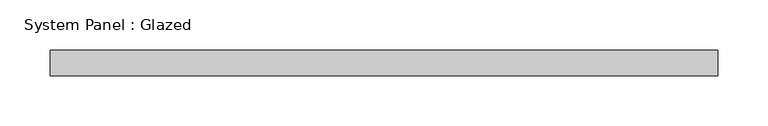
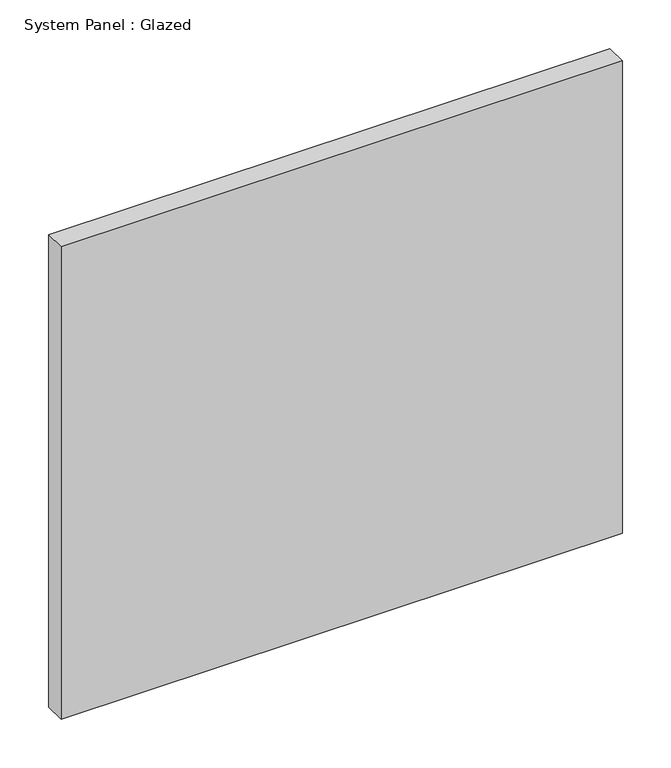
"""IFC4 building model written with IfcOpenShell, lengths in millimetres: plate geometry, System Panel : Glazed."""

from ifc_helpers import new_model, si_unit, origin, origin_with_axes, place, context, project, spatial, polyline, outline, extrude, source, transform, mapped, element, save


def system_panel_glazed_54165e4b(model_context):
    return source(origin(), model_context, "Body", "SweptSolid", [
        extrude(outline(polyline([(333.375, 19.05), (-333.375, 19.05), (-333.375, 44.45), (333.375, 44.45), (333.375, 19.05)])), origin_with_axes(), (0.0, 0.0, 1.0), 592.6666667),
    ])


if __name__ == "__main__":
    model = new_model("IFC4")
    model_context = context("Model", 3, world=origin())
    ifc_project = project(units=[si_unit("LENGTHUNIT", "METRE", prefix="MILLI")], contexts=[model_context])
    site = spatial("IfcSite", under=ifc_project)
    building = spatial("IfcBuilding", under=site)
    placement = place(None, origin())
    system_panel_glazed_shape = system_panel_glazed_54165e4b(model_context)
    element("IfcPlate", 1, ObjectType="System Panel : Glazed", at=placement, inside=building, context=model_context, shape_type="MappedRepresentation", body=[
        mapped(system_panel_glazed_shape, transform((0.0, 0.0, 0.0), x_axis=(1.0, 0.0, 0.0), y_axis=(0.0, 1.0, 0.0), z_axis=(0.0, 0.0, 1.0))),
    ])
    save(model, "model.ifc")

# Revit data of these elements
# Type "System Panel : Glazed"
#   Construction Type Id = "GSP4R"
#   Analytic Construction = "1/8 in Pilkington single glazing"
#   Visual Light Transmittance = 0.9
#   Solar Heat Gain Coefficient = 0.86
#   Heat Transfer Coefficient (U) = 1.18115 BTU/(h·ft²·°F)
#   Define Thermal Properties by = 1
# Element 1 (IfcPlate, "System Panel : Glazed")
#   Materials on its faces: "Glass"
# Materials
#   "Glass": class "Glass", colour RGB 0 128 192, transparency 0.75, Description = "Soda Lime Glass", Cost = 0
